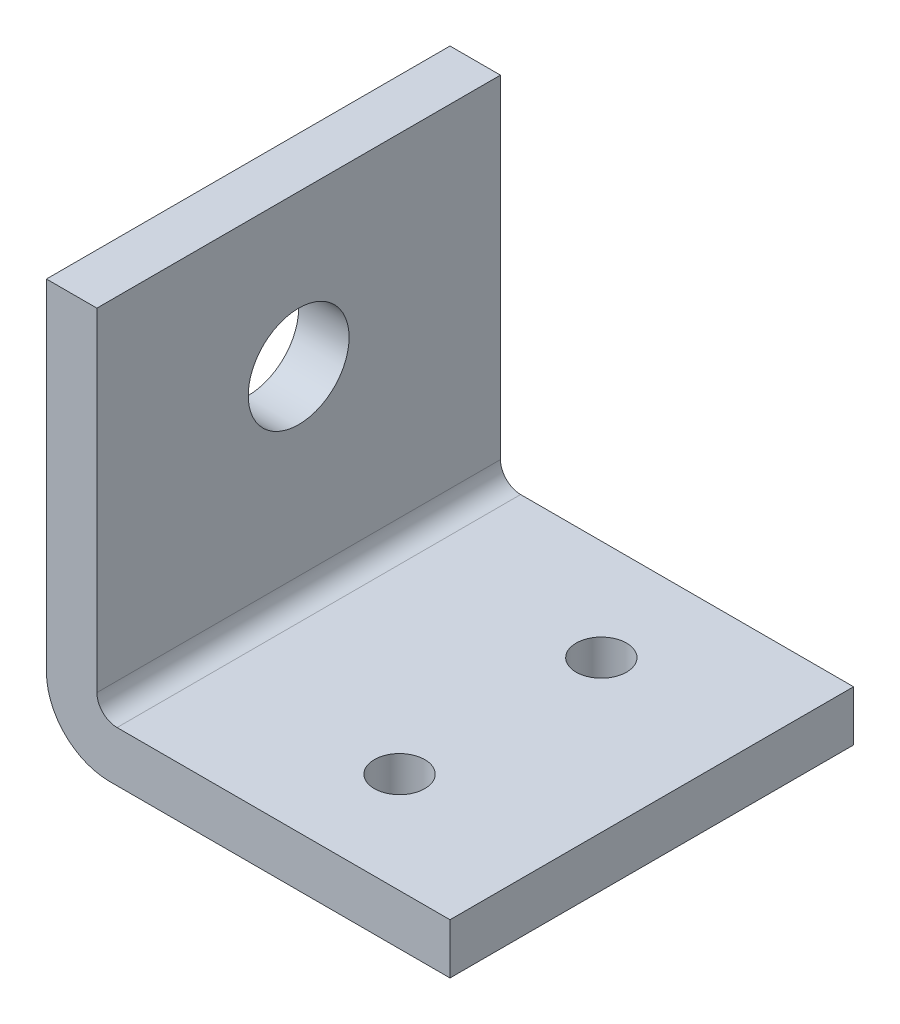
from build123d import *

# Parameters (mm, degrees)
L_BRACKET_BODY_DEPTH  = 20
UPRIGHT_HOLE_SKETCH_R = 5
UPRIGHT_HOLE_10_DEPTH = 57.789083458
BASE_HOLES_SKETCH_R   = 2.5
BASE_HOLES_2X_5_DEPTH = 57.789083458


with BuildPart() as part:
    # Bracket Profile Sketch → L-Bracket Body (new, symmetric)
    with BuildSketch(Plane.XY):
        with BuildLine():
            Line((0, 6.25), (0, 40))
            Line((0, 40), (5, 40))
            Line((5, 40), (5, 7))
            ThreePointArc((5, 7), (5.585786438, 5.585786438), (7, 5))
            Line((7, 5), (40, 5))
            Line((40, 5), (40, 0))
            Line((40, 0), (6.25, 0))
            ThreePointArc((6.25, 0), (1.830582618, 1.830582618), (0, 6.25))
        make_face()
    extrude(amount=L_BRACKET_BODY_DEPTH, both=True)

    # Upright Hole Sketch → Upright Hole Ø10 (cut, through all)
    with BuildSketch(Plane(origin=(5, 0, 0), x_dir=(0, 0, -1), z_dir=(1, 0, 0))):
        with Locations((0, 25)):
            Circle(UPRIGHT_HOLE_SKETCH_R)
    extrude(amount=-UPRIGHT_HOLE_10_DEPTH, mode=Mode.SUBTRACT)

    # Base Holes Sketch → Base Holes 2xØ5 (cut, through all)
    with BuildSketch(Plane(origin=(0, 5, 0), x_dir=(1, 0, 0), z_dir=(0, 1, 0))):
        with Locations(Location((25, 10, 0), (0, 0, 270))):
            Circle(BASE_HOLES_SKETCH_R)
        with Locations(Location((25, -10, 0), (0, 0, 270))):
            Circle(BASE_HOLES_SKETCH_R)
    extrude(amount=-BASE_HOLES_2X_5_DEPTH, mode=Mode.SUBTRACT)


solid = part.part
